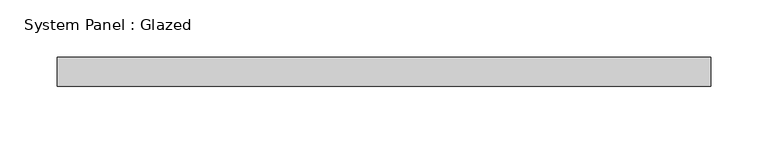
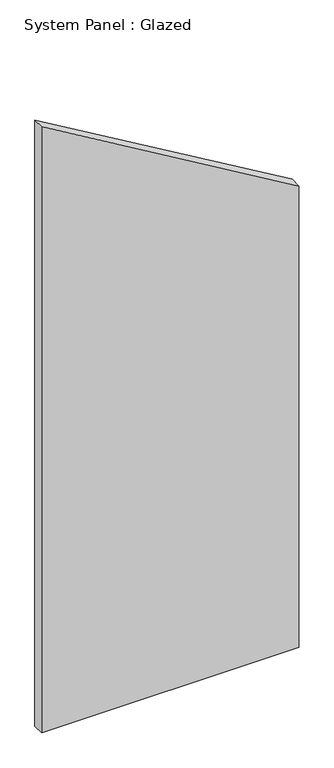
"""IFC4 building model written with IfcOpenShell, lengths in millimetres: plate geometry, System Panel : Glazed."""

from ifc_helpers import new_model, si_unit, frame, origin, place, context, project, spatial, polyline, outline, extrude, source, transform, mapped, element, save


def system_panel_glazed_0f57d06b(model_context):
    return source(origin(), model_context, "Body", "SweptSolid", [
        extrude(outline(polyline([(0.0, -285.75), (0.0, 285.75), (1085.2676875, 285.75), (1424.9353958, -285.75), (0.0, -285.75)])), frame((0.0, 19.05, 0.0), z_axis=(0.0, 1.0, 0.0), x_axis=(0.0, 0.0, 1.0)), (0.0, 0.0, 1.0), 25.4),
    ])


if __name__ == "__main__":
    model = new_model("IFC4")
    model_context = context("Model", 3, world=origin())
    ifc_project = project(units=[si_unit("LENGTHUNIT", "METRE", prefix="MILLI")], contexts=[model_context])
    site = spatial("IfcSite", under=ifc_project)
    building = spatial("IfcBuilding", under=site)
    placement = place(None, origin())
    system_panel_glazed_shape = system_panel_glazed_0f57d06b(model_context)
    element("IfcPlate", 1, ObjectType="System Panel : Glazed", at=placement, inside=building, context=model_context, shape_type="MappedRepresentation", body=[
        mapped(system_panel_glazed_shape, transform((0.0, 0.0, 0.0), x_axis=(1.0, 0.0, 0.0), y_axis=(0.0, 1.0, 0.0), z_axis=(0.0, 0.0, 1.0))),
    ])
    save(model, "model.ifc")

# Revit data of these elements
# Type "System Panel : Glazed"
#   Construction Type Id = "GSP4R"
#   Analytic Construction = "1/8 in Pilkington single glazing"
#   Visual Light Transmittance = 0.9
#   Solar Heat Gain Coefficient = 0.86
#   Heat Transfer Coefficient (U) = 1.18115 BTU/(h·ft²·°F)
#   Define Thermal Properties by = 1
# Element 1 (IfcPlate, "System Panel : Glazed")
#   Materials on its faces: "Glass"
# Materials
#   "Glass": class "Glass", colour RGB 0 128 192, transparency 0.75, Description = "Soda Lime Glass", Cost = 0
